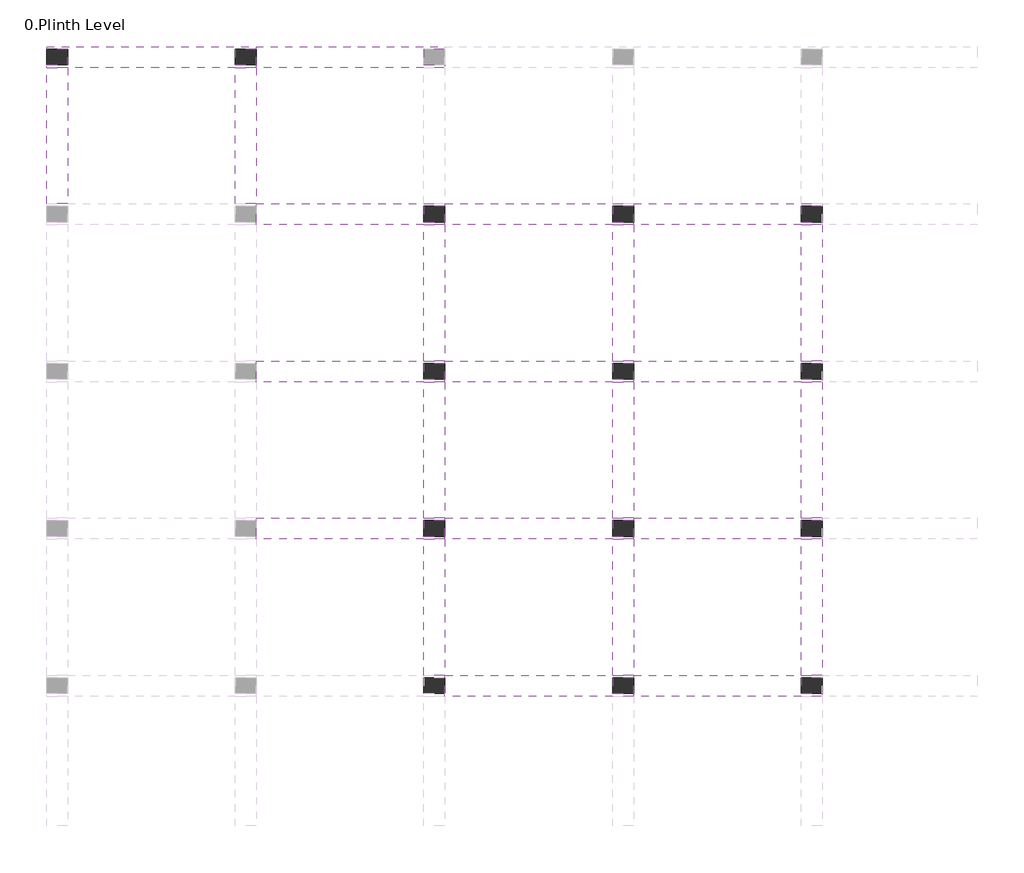
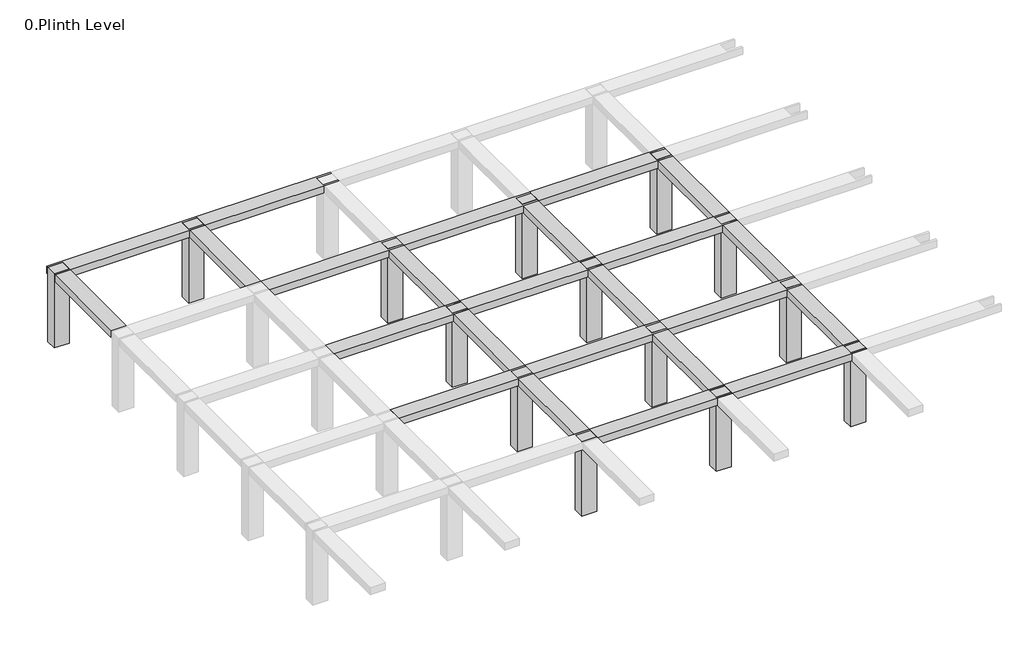
# One storey, part 2 of 3: 24 beams, 14 columns.
"""IFC4 building model written with IfcOpenShell, lengths in millimetres."""

from ifc_helpers import new_model, si_unit, frame, origin, origin_with_axes, place, context, project, spatial, polyline, outline, extrude, faceted_brep, element, save

model = new_model("IFC4")

# Units and contexts
model_context = context("Model", 3, world=origin())
ifc_project = project(units=[si_unit("LENGTHUNIT", "METRE", prefix="MILLI")], contexts=[model_context])

# Site, building, storey
site = spatial("IfcSite", under=ifc_project)
building = spatial("IfcBuilding", under=site)
storey = spatial("IfcBuildingStorey", under=building, Name="0.Plinth Level", Elevation=0.0)

# Beams
placement = place(None, origin())
element("IfcBeam", 1, ObjectType="Concrete-Rectangular Beam : 2' x2'", at=placement, inside=storey, context=model_context, shape_type="Brep", body=[
    faceted_brep([(-5646.474232, 1680.7831222, 3200.4), (-6256.074232, 1680.7831222, 3200.4), (-11132.874232, 1680.7831222, 3200.4), (-11132.874232, 1604.5831222, 3200.4), (-11132.874232, 1147.3831222, 3200.4), (-11132.874232, 1071.1831222, 3200.4), (-6256.074232, 1071.1831222, 3200.4), (-5646.474232, 1071.1831222, 3200.4), (-5646.474232, 1147.3831222, 3200.4), (-6256.074232, 1147.3831222, 3200.4), (-6256.074232, 1604.5831222, 3200.4), (-5646.474232, 1604.5831222, 3200.4), (-5646.474232, 1071.1831222, 2895.6), (-11132.874232, 1071.1831222, 2895.6), (-6256.074232, 1071.1831222, 2895.6), (-11132.874232, 1147.3831222, 2895.6), (-11132.874232, 1604.5831222, 2895.6), (-11132.874232, 1680.7831222, 2895.6), (-6256.074232, 1680.7831222, 2895.6), (-5646.474232, 1680.7831222, 2895.6), (-5646.474232, 1604.5831222, 2895.6), (-6256.074232, 1604.5831222, 2895.6), (-6256.074232, 1147.3831222, 2895.6), (-5646.474232, 1147.3831222, 2895.6)], [[[0, 1, 2, 3, 4, 5, 6, 7, 8, 9, 10, 11]], [[12, 7, 6, 5, 13, 14]], [[12, 14, 13, 15, 16, 17, 18, 19, 20, 21, 22, 23]], [[0, 19, 18, 17, 2, 1]], [[7, 12, 23, 8]], [[5, 4, 3, 2, 17, 16, 15, 13]], [[22, 9, 8, 23]], [[9, 22, 21, 10]], [[10, 21, 20, 11]], [[19, 0, 11, 20]]]),
])
element("IfcBeam", 2, ObjectType="Concrete-Rectangular Beam : 2' x2'", at=placement, inside=storey, context=model_context, shape_type="Brep", body=[
    faceted_brep([(-5646.474232, 1680.7831222, 3200.4), (-5646.474232, 1604.5831222, 3200.4), (-5646.474232, 1147.3831222, 3200.4), (-5646.474232, 1071.1831222, 3200.4), (-769.674232, 1071.1831222, 3200.4), (-160.074232, 1071.1831222, 3200.4), (-160.074232, 1147.3831222, 3200.4), (-769.674232, 1147.3831222, 3200.4), (-769.674232, 1604.5831222, 3200.4), (-160.074232, 1604.5831222, 3200.4), (-160.074232, 1680.7831222, 3200.4), (-769.674232, 1680.7831222, 3200.4), (-5646.474232, 1071.1831222, 2895.6), (-769.674232, 1071.1831222, 2895.6), (-160.074232, 1071.1831222, 2895.6), (-5646.474232, 1147.3831222, 2895.6), (-5646.474232, 1604.5831222, 2895.6), (-5646.474232, 1680.7831222, 2895.6), (-769.674232, 1680.7831222, 2895.6), (-160.074232, 1680.7831222, 2895.6), (-160.074232, 1604.5831222, 2895.6), (-769.674232, 1604.5831222, 2895.6), (-769.674232, 1147.3831222, 2895.6), (-160.074232, 1147.3831222, 2895.6)], [[[0, 1, 2, 3, 4, 5, 6, 7, 8, 9, 10, 11]], [[3, 12, 13, 14, 5, 4]], [[12, 15, 16, 17, 18, 19, 20, 21, 22, 23, 14, 13]], [[10, 19, 18, 17, 0, 11]], [[3, 2, 1, 0, 17, 16, 15, 12]], [[5, 14, 23, 6]], [[22, 7, 6, 23]], [[7, 22, 21, 8]], [[8, 21, 20, 9]], [[19, 10, 9, 20]]]),
])
element("IfcBeam", 3, ObjectType="Concrete-Rectangular Beam : 2' x2'", at=placement, inside=storey, context=model_context, shape_type="Brep", body=[
    faceted_brep([(-16619.274232, 6252.7831222, 3200.4), (-16619.274232, 6176.5831222, 3200.4), (-16619.274232, 5719.3831222, 3200.4), (-16619.274232, 5643.1831222, 3200.4), (-11742.474232, 5643.1831222, 3200.4), (-11132.874232, 5643.1831222, 3200.4), (-11132.874232, 5719.3831222, 3200.4), (-11742.474232, 5719.3831222, 3200.4), (-11742.474232, 6176.5831222, 3200.4), (-11132.874232, 6176.5831222, 3200.4), (-11132.874232, 6252.7831222, 3200.4), (-11742.474232, 6252.7831222, 3200.4), (-16619.274232, 5643.1831222, 2895.6), (-11742.474232, 5643.1831222, 2895.6), (-11132.874232, 5643.1831222, 2895.6), (-16619.274232, 5719.3831222, 2895.6), (-16619.274232, 6176.5831222, 2895.6), (-16619.274232, 6252.7831222, 2895.6), (-11742.474232, 6252.7831222, 2895.6), (-11132.874232, 6252.7831222, 2895.6), (-11132.874232, 6176.5831222, 2895.6), (-11742.474232, 6176.5831222, 2895.6), (-11742.474232, 5719.3831222, 2895.6), (-11132.874232, 5719.3831222, 2895.6)], [[[0, 1, 2, 3, 4, 5, 6, 7, 8, 9, 10, 11]], [[3, 12, 13, 14, 5, 4]], [[12, 15, 16, 17, 18, 19, 20, 21, 22, 23, 14, 13]], [[10, 19, 18, 17, 0, 11]], [[3, 2, 1, 0, 17, 16, 15, 12]], [[5, 14, 23, 6]], [[22, 7, 6, 23]], [[7, 22, 21, 8]], [[8, 21, 20, 9]], [[19, 10, 9, 20]]]),
])
element("IfcBeam", 4, ObjectType="Concrete-Rectangular Beam : 2' x2'", at=placement, inside=storey, context=model_context, shape_type="Brep", body=[
    faceted_brep([(-5646.474232, 6252.7831222, 3200.4), (-6256.074232, 6252.7831222, 3200.4), (-11132.874232, 6252.7831222, 3200.4), (-11132.874232, 6176.5831222, 3200.4), (-11132.874232, 5719.3831222, 3200.4), (-11132.874232, 5643.1831222, 3200.4), (-6256.074232, 5643.1831222, 3200.4), (-5646.474232, 5643.1831222, 3200.4), (-5646.474232, 5719.3831222, 3200.4), (-6256.074232, 5719.3831222, 3200.4), (-6256.074232, 6176.5831222, 3200.4), (-5646.474232, 6176.5831222, 3200.4), (-5646.474232, 5643.1831222, 2895.6), (-11132.874232, 5643.1831222, 2895.6), (-6256.074232, 5643.1831222, 2895.6), (-11132.874232, 5719.3831222, 2895.6), (-11132.874232, 6176.5831222, 2895.6), (-11132.874232, 6252.7831222, 2895.6), (-6256.074232, 6252.7831222, 2895.6), (-5646.474232, 6252.7831222, 2895.6), (-5646.474232, 6176.5831222, 2895.6), (-6256.074232, 6176.5831222, 2895.6), (-6256.074232, 5719.3831222, 2895.6), (-5646.474232, 5719.3831222, 2895.6)], [[[0, 1, 2, 3, 4, 5, 6, 7, 8, 9, 10, 11]], [[12, 7, 6, 5, 13, 14]], [[12, 14, 13, 15, 16, 17, 18, 19, 20, 21, 22, 23]], [[0, 19, 18, 17, 2, 1]], [[7, 12, 23, 8]], [[5, 4, 3, 2, 17, 16, 15, 13]], [[22, 9, 8, 23]], [[9, 22, 21, 10]], [[10, 21, 20, 11]], [[19, 0, 11, 20]]]),
])
element("IfcBeam", 5, ObjectType="Concrete-Rectangular Beam : 2' x2'", at=placement, inside=storey, context=model_context, shape_type="Brep", body=[
    faceted_brep([(-5646.474232, 6252.7831222, 3200.4), (-5646.474232, 6176.5831222, 3200.4), (-5646.474232, 5719.3831222, 3200.4), (-5646.474232, 5643.1831222, 3200.4), (-769.674232, 5643.1831222, 3200.4), (-160.074232, 5643.1831222, 3200.4), (-160.074232, 5719.3831222, 3200.4), (-769.674232, 5719.3831222, 3200.4), (-769.674232, 6176.5831222, 3200.4), (-160.074232, 6176.5831222, 3200.4), (-160.074232, 6252.7831222, 3200.4), (-769.674232, 6252.7831222, 3200.4), (-5646.474232, 5643.1831222, 2895.6), (-769.674232, 5643.1831222, 2895.6), (-160.074232, 5643.1831222, 2895.6), (-5646.474232, 5719.3831222, 2895.6), (-5646.474232, 6176.5831222, 2895.6), (-5646.474232, 6252.7831222, 2895.6), (-769.674232, 6252.7831222, 2895.6), (-160.074232, 6252.7831222, 2895.6), (-160.074232, 6176.5831222, 2895.6), (-769.674232, 6176.5831222, 2895.6), (-769.674232, 5719.3831222, 2895.6), (-160.074232, 5719.3831222, 2895.6)], [[[0, 1, 2, 3, 4, 5, 6, 7, 8, 9, 10, 11]], [[3, 12, 13, 14, 5, 4]], [[12, 15, 16, 17, 18, 19, 20, 21, 22, 23, 14, 13]], [[10, 19, 18, 17, 0, 11]], [[3, 2, 1, 0, 17, 16, 15, 12]], [[5, 14, 23, 6]], [[22, 7, 6, 23]], [[7, 22, 21, 8]], [[8, 21, 20, 9]], [[19, 10, 9, 20]]]),
])
element("IfcBeam", 6, ObjectType="Concrete-Rectangular Beam : 2' x2'", at=placement, inside=storey, context=model_context, shape_type="Brep", body=[
    faceted_brep([(-16619.274232, 10824.7831222, 3200.4), (-16619.274232, 10748.5831222, 3200.4), (-16619.274232, 10291.3831222, 3200.4), (-16619.274232, 10215.1831222, 3200.4), (-11742.474232, 10215.1831222, 3200.4), (-11132.874232, 10215.1831222, 3200.4), (-11132.874232, 10291.3831222, 3200.4), (-11742.474232, 10291.3831222, 3200.4), (-11742.474232, 10748.5831222, 3200.4), (-11132.874232, 10748.5831222, 3200.4), (-11132.874232, 10824.7831222, 3200.4), (-11742.474232, 10824.7831222, 3200.4), (-16619.274232, 10215.1831222, 2895.6), (-11742.474232, 10215.1831222, 2895.6), (-11132.874232, 10215.1831222, 2895.6), (-16619.274232, 10291.3831222, 2895.6), (-16619.274232, 10748.5831222, 2895.6), (-16619.274232, 10824.7831222, 2895.6), (-11742.474232, 10824.7831222, 2895.6), (-11132.874232, 10824.7831222, 2895.6), (-11132.874232, 10748.5831222, 2895.6), (-11742.474232, 10748.5831222, 2895.6), (-11742.474232, 10291.3831222, 2895.6), (-11132.874232, 10291.3831222, 2895.6)], [[[0, 1, 2, 3, 4, 5, 6, 7, 8, 9, 10, 11]], [[3, 12, 13, 14, 5, 4]], [[12, 15, 16, 17, 18, 19, 20, 21, 22, 23, 14, 13]], [[10, 19, 18, 17, 0, 11]], [[3, 2, 1, 0, 17, 16, 15, 12]], [[5, 14, 23, 6]], [[22, 7, 6, 23]], [[7, 22, 21, 8]], [[8, 21, 20, 9]], [[19, 10, 9, 20]]]),
])
element("IfcBeam", 7, ObjectType="Concrete-Rectangular Beam : 2' x2'", at=placement, inside=storey, context=model_context, shape_type="Brep", body=[
    faceted_brep([(-11132.874232, 10824.7831222, 3200.4), (-11132.874232, 10748.5831222, 3200.4), (-11132.874232, 10291.3831222, 3200.4), (-11132.874232, 10215.1831222, 3200.4), (-6256.074232, 10215.1831222, 3200.4), (-5646.474232, 10215.1831222, 3200.4), (-5646.474232, 10291.3831222, 3200.4), (-6256.074232, 10291.3831222, 3200.4), (-6256.074232, 10748.5831222, 3200.4), (-5646.474232, 10748.5831222, 3200.4), (-5646.474232, 10824.7831222, 3200.4), (-6256.074232, 10824.7831222, 3200.4), (-11132.874232, 10215.1831222, 2895.6), (-6256.074232, 10215.1831222, 2895.6), (-5646.474232, 10215.1831222, 2895.6), (-11132.874232, 10291.3831222, 2895.6), (-11132.874232, 10748.5831222, 2895.6), (-11132.874232, 10824.7831222, 2895.6), (-6256.074232, 10824.7831222, 2895.6), (-5646.474232, 10824.7831222, 2895.6), (-5646.474232, 10748.5831222, 2895.6), (-6256.074232, 10748.5831222, 2895.6), (-6256.074232, 10291.3831222, 2895.6), (-5646.474232, 10291.3831222, 2895.6)], [[[0, 1, 2, 3, 4, 5, 6, 7, 8, 9, 10, 11]], [[3, 12, 13, 14, 5, 4]], [[12, 15, 16, 17, 18, 19, 20, 21, 22, 23, 14, 13]], [[10, 19, 18, 17, 0, 11]], [[3, 2, 1, 0, 17, 16, 15, 12]], [[5, 14, 23, 6]], [[22, 7, 6, 23]], [[7, 22, 21, 8]], [[8, 21, 20, 9]], [[19, 10, 9, 20]]]),
])
element("IfcBeam", 8, ObjectType="Concrete-Rectangular Beam : 2' x2'", at=placement, inside=storey, context=model_context, shape_type="Brep", body=[
    faceted_brep([(-5646.474232, 10824.7831222, 3200.4), (-5646.474232, 10748.5831222, 3200.4), (-5646.474232, 10291.3831222, 3200.4), (-5646.474232, 10215.1831222, 3200.4), (-769.674232, 10215.1831222, 3200.4), (-160.074232, 10215.1831222, 3200.4), (-160.074232, 10291.3831222, 3200.4), (-769.674232, 10291.3831222, 3200.4), (-769.674232, 10748.5831222, 3200.4), (-160.074232, 10748.5831222, 3200.4), (-160.074232, 10824.7831222, 3200.4), (-769.674232, 10824.7831222, 3200.4), (-5646.474232, 10215.1831222, 2895.6), (-769.674232, 10215.1831222, 2895.6), (-160.074232, 10215.1831222, 2895.6), (-5646.474232, 10291.3831222, 2895.6), (-5646.474232, 10748.5831222, 2895.6), (-5646.474232, 10824.7831222, 2895.6), (-769.674232, 10824.7831222, 2895.6), (-160.074232, 10824.7831222, 2895.6), (-160.074232, 10748.5831222, 2895.6), (-769.674232, 10748.5831222, 2895.6), (-769.674232, 10291.3831222, 2895.6), (-160.074232, 10291.3831222, 2895.6)], [[[0, 1, 2, 3, 4, 5, 6, 7, 8, 9, 10, 11]], [[3, 12, 13, 14, 5, 4]], [[12, 15, 16, 17, 18, 19, 20, 21, 22, 23, 14, 13]], [[10, 19, 18, 17, 0, 11]], [[3, 2, 1, 0, 17, 16, 15, 12]], [[5, 14, 23, 6]], [[22, 7, 6, 23]], [[7, 22, 21, 8]], [[8, 21, 20, 9]], [[19, 10, 9, 20]]]),
])
element("IfcBeam", 9, ObjectType="Concrete-Rectangular Beam : 2' x2'", at=placement, inside=storey, context=model_context, shape_type="Brep", body=[
    faceted_brep([(-16619.274232, 15396.7831222, 3200.4), (-16619.274232, 15320.5831222, 3200.4), (-16619.274232, 14863.3831222, 3200.4), (-16619.274232, 14787.1831222, 3200.4), (-11742.474232, 14787.1831222, 3200.4), (-11132.874232, 14787.1831222, 3200.4), (-11132.874232, 14863.3831222, 3200.4), (-11742.474232, 14863.3831222, 3200.4), (-11742.474232, 15320.5831222, 3200.4), (-11132.874232, 15320.5831222, 3200.4), (-11132.874232, 15396.7831222, 3200.4), (-11742.474232, 15396.7831222, 3200.4), (-16619.274232, 14787.1831222, 2895.6), (-11742.474232, 14787.1831222, 2895.6), (-11132.874232, 14787.1831222, 2895.6), (-16619.274232, 14863.3831222, 2895.6), (-16619.274232, 15320.5831222, 2895.6), (-16619.274232, 15396.7831222, 2895.6), (-11742.474232, 15396.7831222, 2895.6), (-11132.874232, 15396.7831222, 2895.6), (-11132.874232, 15320.5831222, 2895.6), (-11742.474232, 15320.5831222, 2895.6), (-11742.474232, 14863.3831222, 2895.6), (-11132.874232, 14863.3831222, 2895.6)], [[[0, 1, 2, 3, 4, 5, 6, 7, 8, 9, 10, 11]], [[3, 12, 13, 14, 5, 4]], [[12, 15, 16, 17, 18, 19, 20, 21, 22, 23, 14, 13]], [[10, 19, 18, 17, 0, 11]], [[3, 2, 1, 0, 17, 16, 15, 12]], [[5, 14, 23, 6]], [[22, 7, 6, 23]], [[7, 22, 21, 8]], [[8, 21, 20, 9]], [[19, 10, 9, 20]]]),
])
element("IfcBeam", 10, ObjectType="Concrete-Rectangular Beam : 2' x2'", at=placement, inside=storey, context=model_context, shape_type="Brep", body=[
    faceted_brep([(-11132.874232, 15396.7831222, 3200.4), (-11132.874232, 15320.5831222, 3200.4), (-11132.874232, 14863.3831222, 3200.4), (-11132.874232, 14787.1831222, 3200.4), (-6256.074232, 14787.1831222, 3200.4), (-5646.474232, 14787.1831222, 3200.4), (-5646.474232, 14863.3831222, 3200.4), (-6256.074232, 14863.3831222, 3200.4), (-6256.074232, 15320.5831222, 3200.4), (-5646.474232, 15320.5831222, 3200.4), (-5646.474232, 15396.7831222, 3200.4), (-6256.074232, 15396.7831222, 3200.4), (-11132.874232, 14787.1831222, 2895.6), (-6256.074232, 14787.1831222, 2895.6), (-5646.474232, 14787.1831222, 2895.6), (-11132.874232, 14863.3831222, 2895.6), (-11132.874232, 15320.5831222, 2895.6), (-11132.874232, 15396.7831222, 2895.6), (-6256.074232, 15396.7831222, 2895.6), (-5646.474232, 15396.7831222, 2895.6), (-5646.474232, 15320.5831222, 2895.6), (-6256.074232, 15320.5831222, 2895.6), (-6256.074232, 14863.3831222, 2895.6), (-5646.474232, 14863.3831222, 2895.6)], [[[0, 1, 2, 3, 4, 5, 6, 7, 8, 9, 10, 11]], [[3, 12, 13, 14, 5, 4]], [[12, 15, 16, 17, 18, 19, 20, 21, 22, 23, 14, 13]], [[10, 19, 18, 17, 0, 11]], [[3, 2, 1, 0, 17, 16, 15, 12]], [[5, 14, 23, 6]], [[22, 7, 6, 23]], [[7, 22, 21, 8]], [[8, 21, 20, 9]], [[19, 10, 9, 20]]]),
])
element("IfcBeam", 11, ObjectType="Concrete-Rectangular Beam : 2' x2'", at=placement, inside=storey, context=model_context, shape_type="Brep", body=[
    faceted_brep([(-5646.474232, 15396.7831222, 3200.4), (-5646.474232, 15320.5831222, 3200.4), (-5646.474232, 14863.3831222, 3200.4), (-5646.474232, 14787.1831222, 3200.4), (-769.674232, 14787.1831222, 3200.4), (-160.074232, 14787.1831222, 3200.4), (-160.074232, 14863.3831222, 3200.4), (-769.674232, 14863.3831222, 3200.4), (-769.674232, 15320.5831222, 3200.4), (-160.074232, 15320.5831222, 3200.4), (-160.074232, 15396.7831222, 3200.4), (-769.674232, 15396.7831222, 3200.4), (-5646.474232, 14787.1831222, 2895.6), (-769.674232, 14787.1831222, 2895.6), (-160.074232, 14787.1831222, 2895.6), (-5646.474232, 14863.3831222, 2895.6), (-5646.474232, 15320.5831222, 2895.6), (-5646.474232, 15396.7831222, 2895.6), (-769.674232, 15396.7831222, 2895.6), (-160.074232, 15396.7831222, 2895.6), (-160.074232, 15320.5831222, 2895.6), (-769.674232, 15320.5831222, 2895.6), (-769.674232, 14863.3831222, 2895.6), (-160.074232, 14863.3831222, 2895.6)], [[[0, 1, 2, 3, 4, 5, 6, 7, 8, 9, 10, 11]], [[3, 12, 13, 14, 5, 4]], [[12, 15, 16, 17, 18, 19, 20, 21, 22, 23, 14, 13]], [[10, 19, 18, 17, 0, 11]], [[3, 2, 1, 0, 17, 16, 15, 12]], [[5, 14, 23, 6]], [[22, 7, 6, 23]], [[7, 22, 21, 8]], [[8, 21, 20, 9]], [[19, 10, 9, 20]]]),
])
element("IfcBeam", 12, ObjectType="Concrete-Rectangular Beam : 2' x2'", at=placement, inside=storey, context=model_context, shape_type="Brep", body=[
    faceted_brep([(-16619.274232, 19968.7831222, 3200.4), (-22715.274232, 19968.7831222, 3200.4), (-22715.274232, 19892.5831222, 3200.4), (-22105.674232, 19892.5831222, 3200.4), (-22105.674232, 19435.3831222, 3200.4), (-22715.274232, 19435.3831222, 3200.4), (-22715.274232, 19359.1831222, 3200.4), (-22105.674232, 19359.1831222, 3200.4), (-17228.874232, 19359.1831222, 3200.4), (-16619.274232, 19359.1831222, 3200.4), (-16619.274232, 19435.3831222, 3200.4), (-17228.874232, 19435.3831222, 3200.4), (-17228.874232, 19892.5831222, 3200.4), (-16619.274232, 19892.5831222, 3200.4), (-22715.274232, 19359.1831222, 2895.6), (-22105.674232, 19359.1831222, 2895.6), (-17228.874232, 19359.1831222, 2895.6), (-16619.274232, 19359.1831222, 2895.6), (-22715.274232, 19435.3831222, 2895.6), (-22105.674232, 19435.3831222, 2895.6), (-22105.674232, 19892.5831222, 2895.6), (-22715.274232, 19892.5831222, 2895.6), (-22715.274232, 19968.7831222, 2895.6), (-16619.274232, 19968.7831222, 2895.6), (-16619.274232, 19892.5831222, 2895.6), (-17228.874232, 19892.5831222, 2895.6), (-17228.874232, 19435.3831222, 2895.6), (-16619.274232, 19435.3831222, 2895.6)], [[[0, 1, 2, 3, 4, 5, 6, 7, 8, 9, 10, 11, 12, 13]], [[6, 14, 15, 16, 17, 9, 8, 7]], [[17, 16, 15, 14, 18, 19, 20, 21, 22, 23, 24, 25, 26, 27]], [[22, 1, 0, 23]], [[14, 6, 5, 18]], [[9, 17, 27, 10]], [[19, 4, 3, 20]], [[4, 19, 18, 5]], [[20, 3, 2, 21]], [[1, 22, 21, 2]], [[26, 11, 10, 27]], [[11, 26, 25, 12]], [[12, 25, 24, 13]], [[23, 0, 13, 24]]]),
])
element("IfcBeam", 13, ObjectType="Concrete-Rectangular Beam : 2' x2'", at=placement, inside=storey, context=model_context, shape_type="Brep", body=[
    faceted_brep([(-11132.874232, 19968.7831222, 3200.4), (-16619.274232, 19968.7831222, 3200.4), (-16619.274232, 19892.5831222, 3200.4), (-16619.274232, 19435.3831222, 3200.4), (-16619.274232, 19359.1831222, 3200.4), (-11742.474232, 19359.1831222, 3200.4), (-11132.874232, 19359.1831222, 3200.4), (-11132.874232, 19435.3831222, 3200.4), (-11742.474232, 19435.3831222, 3200.4), (-11742.474232, 19892.5831222, 3200.4), (-11132.874232, 19892.5831222, 3200.4), (-11132.874232, 19359.1831222, 2895.6), (-16619.274232, 19359.1831222, 2895.6), (-11742.474232, 19359.1831222, 2895.6), (-16619.274232, 19435.3831222, 2895.6), (-16619.274232, 19892.5831222, 2895.6), (-16619.274232, 19968.7831222, 2895.6), (-11132.874232, 19968.7831222, 2895.6), (-11132.874232, 19892.5831222, 2895.6), (-11742.474232, 19892.5831222, 2895.6), (-11742.474232, 19435.3831222, 2895.6), (-11132.874232, 19435.3831222, 2895.6)], [[[0, 1, 2, 3, 4, 5, 6, 7, 8, 9, 10]], [[11, 6, 5, 4, 12, 13]], [[11, 13, 12, 14, 15, 16, 17, 18, 19, 20, 21]], [[0, 17, 16, 1]], [[6, 11, 21, 7]], [[4, 3, 2, 1, 16, 15, 14, 12]], [[20, 8, 7, 21]], [[8, 20, 19, 9]], [[9, 19, 18, 10]], [[17, 0, 10, 18]]]),
])
element("IfcBeam", 14, ObjectType="Concrete-Rectangular Beam : 2' x2'", at=placement, inside=storey, context=model_context, shape_type="SweptSolid", body=[
    extrude(outline(polyline([(-22105.674232, 15396.7831222), (-22715.274232, 15396.7831222), (-22715.274232, 19359.1831222), (-22105.674232, 19359.1831222), (-22105.674232, 15396.7831222)])), frame((0.0, 0.0, 2895.6), z_axis=(0.0, 0.0, 1.0), x_axis=(1.0, 0.0, 0.0)), (0.0, 0.0, 1.0), 304.8),
])
element("IfcBeam", 15, ObjectType="Concrete-Rectangular Beam : 2' x2'", at=placement, inside=storey, context=model_context, shape_type="SweptSolid", body=[
    extrude(outline(polyline([(-16619.274232, 15396.7831222), (-17228.874232, 15396.7831222), (-17228.874232, 19359.1831222), (-16619.274232, 19359.1831222), (-16619.274232, 15396.7831222)])), frame((0.0, 0.0, 2895.6), z_axis=(0.0, 0.0, 1.0), x_axis=(1.0, 0.0, 0.0)), (0.0, 0.0, 1.0), 304.8),
])
element("IfcBeam", 16, ObjectType="Concrete-Rectangular Beam : 2' x2'", at=placement, inside=storey, context=model_context, shape_type="SweptSolid", body=[
    extrude(outline(polyline([(-11132.874232, 1680.7831222), (-11742.474232, 1680.7831222), (-11742.474232, 5643.1831222), (-11132.874232, 5643.1831222), (-11132.874232, 1680.7831222)])), frame((0.0, 0.0, 2895.6), z_axis=(0.0, 0.0, 1.0), x_axis=(1.0, 0.0, 0.0)), (0.0, 0.0, 1.0), 304.8),
])
element("IfcBeam", 17, ObjectType="Concrete-Rectangular Beam : 2' x2'", at=placement, inside=storey, context=model_context, shape_type="SweptSolid", body=[
    extrude(outline(polyline([(-11132.874232, 6252.7831222), (-11742.474232, 6252.7831222), (-11742.474232, 10215.1831222), (-11132.874232, 10215.1831222), (-11132.874232, 6252.7831222)])), frame((0.0, 0.0, 2895.6), z_axis=(0.0, 0.0, 1.0), x_axis=(1.0, 0.0, 0.0)), (0.0, 0.0, 1.0), 304.8),
])
element("IfcBeam", 18, ObjectType="Concrete-Rectangular Beam : 2' x2'", at=placement, inside=storey, context=model_context, shape_type="SweptSolid", body=[
    extrude(outline(polyline([(-11132.874232, 10824.7831222), (-11742.474232, 10824.7831222), (-11742.474232, 14787.1831222), (-11132.874232, 14787.1831222), (-11132.874232, 10824.7831222)])), frame((0.0, 0.0, 2895.6), z_axis=(0.0, 0.0, 1.0), x_axis=(1.0, 0.0, 0.0)), (0.0, 0.0, 1.0), 304.8),
])
element("IfcBeam", 19, ObjectType="Concrete-Rectangular Beam : 2' x2'", at=placement, inside=storey, context=model_context, shape_type="SweptSolid", body=[
    extrude(outline(polyline([(-5646.474232, 1680.7831222), (-6256.074232, 1680.7831222), (-6256.074232, 5643.1831222), (-5646.474232, 5643.1831222), (-5646.474232, 1680.7831222)])), frame((0.0, 0.0, 2895.6), z_axis=(0.0, 0.0, 1.0), x_axis=(1.0, 0.0, 0.0)), (0.0, 0.0, 1.0), 304.8),
])
element("IfcBeam", 20, ObjectType="Concrete-Rectangular Beam : 2' x2'", at=placement, inside=storey, context=model_context, shape_type="SweptSolid", body=[
    extrude(outline(polyline([(-5646.474232, 6252.7831222), (-6256.074232, 6252.7831222), (-6256.074232, 10215.1831222), (-5646.474232, 10215.1831222), (-5646.474232, 6252.7831222)])), frame((0.0, 0.0, 2895.6), z_axis=(0.0, 0.0, 1.0), x_axis=(1.0, 0.0, 0.0)), (0.0, 0.0, 1.0), 304.8),
])
element("IfcBeam", 21, ObjectType="Concrete-Rectangular Beam : 2' x2'", at=placement, inside=storey, context=model_context, shape_type="SweptSolid", body=[
    extrude(outline(polyline([(-5646.474232, 10824.7831222), (-6256.074232, 10824.7831222), (-6256.074232, 14787.1831222), (-5646.474232, 14787.1831222), (-5646.474232, 10824.7831222)])), frame((0.0, 0.0, 2895.6), z_axis=(0.0, 0.0, 1.0), x_axis=(1.0, 0.0, 0.0)), (0.0, 0.0, 1.0), 304.8),
])
element("IfcBeam", 22, ObjectType="Concrete-Rectangular Beam : 2' x2'", at=placement, inside=storey, context=model_context, shape_type="SweptSolid", body=[
    extrude(outline(polyline([(-769.674232, 5643.1831222), (-160.074232, 5643.1831222), (-160.074232, 1680.7831222), (-769.674232, 1680.7831222), (-769.674232, 5643.1831222)])), frame((0.0, 0.0, 2895.6), z_axis=(0.0, 0.0, 1.0), x_axis=(1.0, 0.0, 0.0)), (0.0, 0.0, 1.0), 304.8),
])
element("IfcBeam", 23, ObjectType="Concrete-Rectangular Beam : 2' x2'", at=placement, inside=storey, context=model_context, shape_type="SweptSolid", body=[
    extrude(outline(polyline([(-160.074232, 6252.7831222), (-769.674232, 6252.7831222), (-769.674232, 10215.1831222), (-160.074232, 10215.1831222), (-160.074232, 6252.7831222)])), frame((0.0, 0.0, 2895.6), z_axis=(0.0, 0.0, 1.0), x_axis=(1.0, 0.0, 0.0)), (0.0, 0.0, 1.0), 304.8),
])
element("IfcBeam", 24, ObjectType="Concrete-Rectangular Beam : 2' x2'", at=placement, inside=storey, context=model_context, shape_type="SweptSolid", body=[
    extrude(outline(polyline([(-769.674232, 14787.1831222), (-160.074232, 14787.1831222), (-160.074232, 10824.7831222), (-769.674232, 10824.7831222), (-769.674232, 14787.1831222)])), frame((0.0, 0.0, 2895.6), z_axis=(0.0, 0.0, 1.0), x_axis=(1.0, 0.0, 0.0)), (0.0, 0.0, 1.0), 304.8),
])

# Columns
element("IfcColumn", 25, ObjectType="Concrete-Rectangular-Column : 12 x 18", at=placement, inside=storey, context=model_context, shape_type="SweptSolid", body=[
    extrude(outline(polyline([(-11132.874232, 1604.5831222), (-11132.874232, 1147.3831222), (-11742.474232, 1147.3831222), (-11742.474232, 1604.5831222), (-11132.874232, 1604.5831222)])), origin_with_axes(), (0.0, 0.0, 1.0), 3200.4),
])
element("IfcColumn", 26, ObjectType="Concrete-Rectangular-Column : 12 x 18", at=placement, inside=storey, context=model_context, shape_type="SweptSolid", body=[
    extrude(outline(polyline([(-5646.474232, 1604.5831222), (-5646.474232, 1147.3831222), (-6256.074232, 1147.3831222), (-6256.074232, 1604.5831222), (-5646.474232, 1604.5831222)])), origin_with_axes(), (0.0, 0.0, 1.0), 3200.4),
])
element("IfcColumn", 27, ObjectType="Concrete-Rectangular-Column : 12 x 18", at=placement, inside=storey, context=model_context, shape_type="SweptSolid", body=[
    extrude(outline(polyline([(-160.074232, 1604.5831222), (-160.074232, 1147.3831222), (-769.674232, 1147.3831222), (-769.674232, 1604.5831222), (-160.074232, 1604.5831222)])), origin_with_axes(), (0.0, 0.0, 1.0), 3200.4),
])
element("IfcColumn", 28, ObjectType="Concrete-Rectangular-Column : 12 x 18", at=placement, inside=storey, context=model_context, shape_type="SweptSolid", body=[
    extrude(outline(polyline([(-11132.874232, 6176.5831222), (-11132.874232, 5719.3831222), (-11742.474232, 5719.3831222), (-11742.474232, 6176.5831222), (-11132.874232, 6176.5831222)])), origin_with_axes(), (0.0, 0.0, 1.0), 3200.4),
])
element("IfcColumn", 29, ObjectType="Concrete-Rectangular-Column : 12 x 18", at=placement, inside=storey, context=model_context, shape_type="SweptSolid", body=[
    extrude(outline(polyline([(-5646.474232, 6176.5831222), (-5646.474232, 5719.3831222), (-6256.074232, 5719.3831222), (-6256.074232, 6176.5831222), (-5646.474232, 6176.5831222)])), origin_with_axes(), (0.0, 0.0, 1.0), 3200.4),
])
element("IfcColumn", 30, ObjectType="Concrete-Rectangular-Column : 12 x 18", at=placement, inside=storey, context=model_context, shape_type="SweptSolid", body=[
    extrude(outline(polyline([(-160.074232, 6176.5831222), (-160.074232, 5719.3831222), (-769.674232, 5719.3831222), (-769.674232, 6176.5831222), (-160.074232, 6176.5831222)])), origin_with_axes(), (0.0, 0.0, 1.0), 3200.4),
])
element("IfcColumn", 31, ObjectType="Concrete-Rectangular-Column : 12 x 18", at=placement, inside=storey, context=model_context, shape_type="SweptSolid", body=[
    extrude(outline(polyline([(-11132.874232, 10748.5831222), (-11132.874232, 10291.3831222), (-11742.474232, 10291.3831222), (-11742.474232, 10748.5831222), (-11132.874232, 10748.5831222)])), origin_with_axes(), (0.0, 0.0, 1.0), 3200.4),
])
element("IfcColumn", 32, ObjectType="Concrete-Rectangular-Column : 12 x 18", at=placement, inside=storey, context=model_context, shape_type="SweptSolid", body=[
    extrude(outline(polyline([(-5646.474232, 10748.5831222), (-5646.474232, 10291.3831222), (-6256.074232, 10291.3831222), (-6256.074232, 10748.5831222), (-5646.474232, 10748.5831222)])), origin_with_axes(), (0.0, 0.0, 1.0), 3200.4),
])
element("IfcColumn", 33, ObjectType="Concrete-Rectangular-Column : 12 x 18", at=placement, inside=storey, context=model_context, shape_type="SweptSolid", body=[
    extrude(outline(polyline([(-160.074232, 10748.5831222), (-160.074232, 10291.3831222), (-769.674232, 10291.3831222), (-769.674232, 10748.5831222), (-160.074232, 10748.5831222)])), origin_with_axes(), (0.0, 0.0, 1.0), 3200.4),
])
element("IfcColumn", 34, ObjectType="Concrete-Rectangular-Column : 12 x 18", at=placement, inside=storey, context=model_context, shape_type="SweptSolid", body=[
    extrude(outline(polyline([(-11132.874232, 15320.5831222), (-11132.874232, 14863.3831222), (-11742.474232, 14863.3831222), (-11742.474232, 15320.5831222), (-11132.874232, 15320.5831222)])), origin_with_axes(), (0.0, 0.0, 1.0), 3200.4),
])
element("IfcColumn", 35, ObjectType="Concrete-Rectangular-Column : 12 x 18", at=placement, inside=storey, context=model_context, shape_type="SweptSolid", body=[
    extrude(outline(polyline([(-5646.474232, 15320.5831222), (-5646.474232, 14863.3831222), (-6256.074232, 14863.3831222), (-6256.074232, 15320.5831222), (-5646.474232, 15320.5831222)])), origin_with_axes(), (0.0, 0.0, 1.0), 3200.4),
])
element("IfcColumn", 36, ObjectType="Concrete-Rectangular-Column : 12 x 18", at=placement, inside=storey, context=model_context, shape_type="SweptSolid", body=[
    extrude(outline(polyline([(-160.074232, 15320.5831222), (-160.074232, 14863.3831222), (-769.674232, 14863.3831222), (-769.674232, 15320.5831222), (-160.074232, 15320.5831222)])), origin_with_axes(), (0.0, 0.0, 1.0), 3200.4),
])
element("IfcColumn", 37, ObjectType="Concrete-Rectangular-Column : 12 x 18", at=placement, inside=storey, context=model_context, shape_type="SweptSolid", body=[
    extrude(outline(polyline([(-22105.674232, 19892.5831222), (-22105.674232, 19435.3831222), (-22715.274232, 19435.3831222), (-22715.274232, 19892.5831222), (-22105.674232, 19892.5831222)])), origin_with_axes(), (0.0, 0.0, 1.0), 3200.4),
])
element("IfcColumn", 38, ObjectType="Concrete-Rectangular-Column : 12 x 18", at=placement, inside=storey, context=model_context, shape_type="SweptSolid", body=[
    extrude(outline(polyline([(-16619.274232, 19892.5831222), (-16619.274232, 19435.3831222), (-17228.874232, 19435.3831222), (-17228.874232, 19892.5831222), (-16619.274232, 19892.5831222)])), origin_with_axes(), (0.0, 0.0, 1.0), 3200.4),
])

save(model, "model.ifc")

# Revit data of these elements
# Type "Concrete-Rectangular Beam : 2' x2'"
#   Assembly Code = "B10"
#   Length [instance default] = 5' - 0"
#   b = 2' - 0"
#   h = 1' - 0"
#   Structural Material [instance default] = Concrete, Cast-in-Place gray
# Type "Concrete-Rectangular-Column : 12 x 18"
#   Assembly Code = "B10"
#   b = 2' - 0"
#   h = 1' - 6"
#   Structural Material [instance default] = Concrete, Cast-in-Place gray
# Elements 1, 2, 3, 4, 5, 6, 7, 8, 9, 10, 11, 12, 13, 14, 15, 16, 17, 18, 19, 20, 21, 22, 23, 24 (IfcBeam, "Concrete-Rectangular Beam : 2' x2'")
#   Structural Material = Concrete, Precast (2)
#   Phase Created = New Construction
#   Materials on its faces: "Concrete, Precast (2)"
# Elements 25, 26, 27, 28, 29, 30, 31, 32, 33, 34, 35, 36, 37, 38 (IfcColumn, "Concrete-Rectangular-Column : 12 x 18")
#   Phase Created = New Construction
#   Materials on its faces: "Concrete, Cast-in-Place gray"
# Materials
#   "Concrete, Cast-in-Place gray": class "Concrete", colour RGB 192 192 192, transparency 0, Description = "Cast-in-place concrete", Cost = 0
#   "Concrete, Precast (2)": class "Concrete", colour RGB 198 187 187, transparency 0, Description = "Precast concrete", Cost = 0
